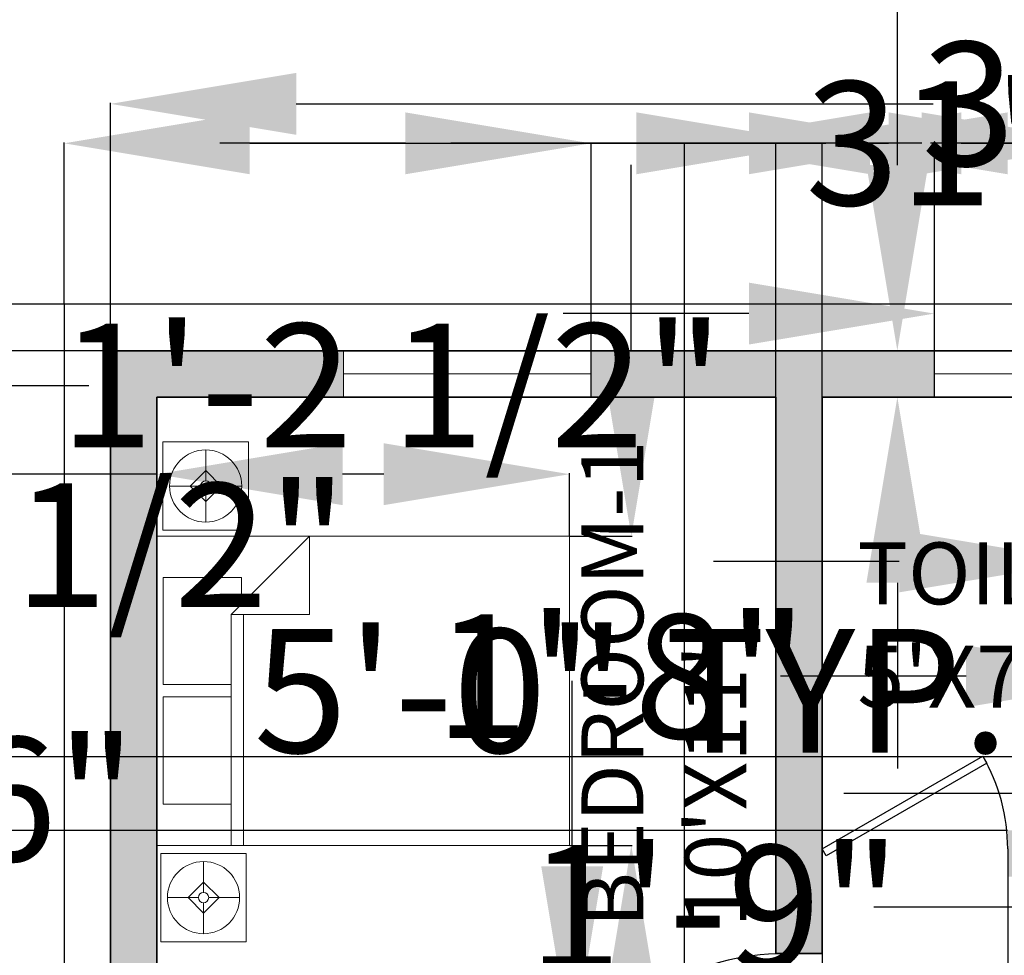
# Model space of a CAD drawing. Units: inches. Extents: x 2838 to 4029, y 1041 to 1915.
# Tile 7 of 16: x 3250 to 3441, y 1554 to 1735. Entities that reach past the tile are written whole.
import ezdxf

# ---------------------------------------------------------------- set-up
doc = ezdxf.new("R2010")
doc.units = ezdxf.units.IN
doc.header["$MEASUREMENT"] = 0
for name, color, linetype, lineweight in [('A-ANNO-DIMS', 2, 'Continuous', 18), ('A-AREA-IDEN', 7, 'Continuous', 18), ('A-DOOR', 3, 'Continuous', 25), ('A-FLOR', 7, 'Continuous', 25), ('A-FURN', 8, 'Continuous', 18), ('A-GLAZ', 4, 'Continuous', 18), ('A-REFR', 8, 'Continuous', 13), ('A-WALL', 7, 'Continuous', 35), ('A-WALL-PATT', 252, 'Continuous', 13)]:
    doc.layers.add(name, color=color, linetype=linetype, lineweight=lineweight)
doc.styles.get("Standard").update_dxf_attribs({"font": 'arial.ttf'})
doc.dimstyles.get("Standard").update_dxf_attribs({"dimtxt": 24, "dimasz": 36, "dimexe": 0.18, "dimexo": 0.0625, "dimgap": 0.09, "dimtad": 0, "dimtih": 1, "dimtoh": 1, "dimdec": 0, "dimzin": 0, "dimdsep": 46, "dimlunit": 3, "dimtxsty": 'Standard', "dimcen": 0.09, "dimadec": 0, "dimazin": 0, "dimtfac": 1, "dimtdec": 0, "dimtofl": 0, "dimtmove": 0, "dimatfit": 3, "dimfxl": 1, "dimtolj": 1, "dimtzin": 0, "dimarcsym": 0})

# ---------------------------------------------------------------- blocks, each defined once
blk = doc.blocks.new('*U2')
for p, q in [((0, 0), (0, -6)), ((40, 0), (40, -6))]:
    blk.add_line(p, q)
blk.add_lwpolyline([(0, 0), (34.64, 20), (35.52, 18.48), (0.87, -1.52)], close=True)
blk.add_arc((0, 0), 40, 0, 30)
blk = doc.blocks.new('*U3')
for p, q in [((-40, 0), (-40, 6)), ((0, 0), (0, 6))]:
    blk.add_line(p, q)
blk.add_lwpolyline([(0, 0), (-20, -34.64), (-21.52, -33.77), (-1.52, 0.88)], close=True)
blk.add_arc((0, 0), 40, 180, 240)
blk = doc.blocks.new('Bed - Queen')
for p, q in [((0, -80.00003), (0, 0)), ((0, 0), (59.99999, 0)), ((59.99999, 0), (59.99999, -80.00003)), ((7.99999, -1.2), (28.79998, -1.2)), ((7.99999, -14.4), (7.99999, -1.2)), ((28.79998, -1.2), (28.79998, -14.4)), ((31.19999, -1.2), (51.99999, -1.2)), ((31.19999, -14.4), (31.19999, -1.2)), ((51.99999, -1.2), (51.99999, -16.4)), ((0, -14.4), (44.8, -14.4)), ((59.99999, -29.6), (44.8, -14.4)), ((44.8, -14.4), (44.8, -29.6)), ((44.8, -16.8), (0, -16.8)), ((51.99999, -16.4), (46.79936, -16.4)), ((44.8, -29.6), (59.99999, -29.6)), ((59.99999, -80.00003), (0, -80.00003))]:
    blk.add_line(p, q)
blk = doc.blocks.new('*D18')
at = {"layer": 'A-ANNO-DIMS', "color": 0, "lineweight": -2, "transparency": 16777216}
for p, q in [((3267.73, 1671.36), (3267.73, 1719.35)), ((3303.73, 1719.17), (3427.28, 1719.17)), ((3591.73, 1719.17), (3468.18, 1719.17)), ((3627.73, 1671.36), (3627.73, 1719.35))]:
    blk.add_line(p, q, dxfattribs=at)
at = {"layer": 'A-ANNO-DIMS', "color": 0, "transparency": 16777216}
for points in [[(3303.73, 1725.17), (3303.73, 1713.17), (3267.73, 1719.17)], [(3591.73, 1725.17), (3591.73, 1713.17), (3627.73, 1719.17)]]:
    blk.add_solid(points, dxfattribs=at)
at = {"layer": 'Defpoints', "color": 0, "transparency": 16777216}
for p in [(3267.73, 1719.17), (3267.73, 1671.3), (3627.73, 1671.3)]:
    blk.add_point(p, dxfattribs=at)
at = {"layer": 'A-ANNO-DIMS', "color": 0, "transparency": 16777216, "insert": (3447.73, 1719.17), "char_height": 24, "attachment_point": 5}
blk.add_mtext("\\A1;30'", dxfattribs=at)
blk = doc.blocks.new('WIN-48')
blk.add_line((4.5, 48), (4.5, 0))
blk.add_lwpolyline([(0, 48), (9, 48), (9, 0), (0, 0)], close=True)
blk = doc.blocks.new('WIN-24-VENT')
for p, q in [((24, 9), (24, 0)), ((24, 4.5), (0, 4.5))]:
    blk.add_line(p, q)
blk.add_lwpolyline([(48, 0), (0, 0), (0, 9), (48, 9)])
blk = doc.blocks.new('Lamp - Table')
for p, q in [((0, 7), (0, 1)), ((0, 3), (-3, 0)), ((3, 0), (0, 3)), ((-1, 0), (-7, 0)), ((-3, 0), (0, -3)), ((0, -3), (3, 0)), ((1, 0), (7, 0)), ((0, -1), (0, -7))]:
    blk.add_line(p, q)
for radius in [7, 1]:
    blk.add_circle((0, 0), radius)
blk = doc.blocks.new('NIGHTSTAND-WITH-LAMP')
blk.add_lwpolyline([(0, 17.15), (16.57, 17.15), (16.57, 0), (0, 0)], close=True)
blk.add_blockref('Lamp - Table', (8.28, 8.57))
blk = doc.blocks.new('*D35')
at = {"layer": 'A-ANNO-DIMS', "color": 0, "lineweight": -2, "transparency": 16777216}
for p, q in [((3480.45, 1632.93), (3480.45, 1668.93)), ((3481.89, 1596.93), (3480.27, 1596.93)), ((3481.89, 1586.93), (3480.27, 1586.93)), ((3480.45, 1550.93), (3480.45, 1514.93)), ((3480.45, 1514.93), (3444.45, 1514.93))]:
    blk.add_line(p, q, dxfattribs=at)
at = {"layer": 'A-ANNO-DIMS', "color": 0, "transparency": 16777216}
for points in [[(3474.45, 1632.93), (3486.45, 1632.93), (3480.45, 1596.93)], [(3474.45, 1550.93), (3486.45, 1550.93), (3480.45, 1586.93)]]:
    blk.add_solid(points, dxfattribs=at)
at = {"layer": 'Defpoints', "color": 0, "transparency": 16777216}
for p in [(3481.95, 1596.93), (3480.45, 1586.93), (3481.95, 1586.93)]:
    blk.add_point(p, dxfattribs=at)
at = {"layer": 'A-ANNO-DIMS', "color": 0, "transparency": 16777216, "insert": (3365.58, 1514.93), "char_height": 24, "attachment_point": 5}
blk.add_mtext('\\A1;TAP 0\'-10"', dxfattribs=at)
blk = doc.blocks.new('*D36')
at = {"layer": 'A-ANNO-DIMS', "color": 0, "lineweight": -2, "transparency": 16777216}
for p, q in [((3481.95, 1586.87), (3481.95, 1585.25)), ((3488.45, 1586.87), (3488.45, 1585.25)), ((3445.95, 1585.43), (3409.95, 1585.43)), ((3524.45, 1585.43), (3560.45, 1585.43))]:
    blk.add_line(p, q, dxfattribs=at)
at = {"layer": 'A-ANNO-DIMS', "color": 0, "transparency": 16777216}
for points in [[(3445.95, 1591.43), (3445.95, 1579.43), (3481.95, 1585.43)], [(3524.45, 1591.43), (3524.45, 1579.43), (3488.45, 1585.43)]]:
    blk.add_solid(points, dxfattribs=at)
at = {"layer": 'Defpoints', "color": 0, "transparency": 16777216}
for p in [(3481.95, 1586.93), (3488.45, 1586.93), (3488.45, 1585.43)]:
    blk.add_point(p, dxfattribs=at)
at = {"layer": 'A-ANNO-DIMS', "color": 0, "transparency": 16777216, "insert": (3620.4, 1585.43), "char_height": 24, "attachment_point": 5}
blk.add_mtext('\\A1;0\'-6 1/2"', dxfattribs=at)
blk = doc.blocks.new('*D37')
at = {"layer": 'A-ANNO-DIMS', "color": 0, "lineweight": -2, "transparency": 16777216}
for p, q in [((3276.73, 1647.36), (3240.73, 1647.36)), ((3276.73, 1635.42), (3276.73, 1647.54)), ((3320.73, 1647.36), (3312.73, 1647.36)), ((3356.73, 1635.42), (3356.73, 1647.54))]:
    blk.add_line(p, q, dxfattribs=at)
at = {"layer": 'A-ANNO-DIMS', "color": 0, "transparency": 16777216}
for points in [[(3312.73, 1653.36), (3312.73, 1641.36), (3276.73, 1647.36)], [(3320.73, 1653.36), (3320.73, 1641.36), (3356.73, 1647.36)]]:
    blk.add_solid(points, dxfattribs=at)
at = {"layer": 'Defpoints', "color": 0, "transparency": 16777216}
for p in [(3276.73, 1647.36), (3276.73, 1635.36), (3356.73, 1635.36)]:
    blk.add_point(p, dxfattribs=at)
at = {"layer": 'A-ANNO-DIMS', "color": 0, "transparency": 16777216, "insert": (3064.12, 1647.36), "char_height": 24, "attachment_point": 5}
blk.add_mtext('\\A1;QUEEN BED 6\'-8" TYP.', dxfattribs=at)
blk = doc.blocks.new('*D38')
at = {"layer": 'A-ANNO-DIMS', "color": 0, "lineweight": -2, "transparency": 16777216}
for p, q in [((3368.73, 1671.36), (3368.73, 1707.36)), ((3356.79, 1635.36), (3368.91, 1635.36)), ((3356.79, 1575.36), (3368.91, 1575.36)), ((3368.73, 1539.36), (3368.73, 1503.36))]:
    blk.add_line(p, q, dxfattribs=at)
at = {"layer": 'A-ANNO-DIMS', "color": 0, "transparency": 16777216}
for points in [[(3362.73, 1671.36), (3374.73, 1671.36), (3368.73, 1635.36)], [(3362.73, 1539.36), (3374.73, 1539.36), (3368.73, 1575.36)]]:
    blk.add_solid(points, dxfattribs=at)
at = {"layer": 'Defpoints', "color": 0, "transparency": 16777216}
for p in [(3356.73, 1635.36), (3368.73, 1635.36), (3356.73, 1575.36)]:
    blk.add_point(p, dxfattribs=at)
at = {"layer": 'A-ANNO-DIMS', "color": 0, "transparency": 16777216, "insert": (3368.73, 1605.36), "char_height": 24, "attachment_point": 5}
blk.add_mtext('\\A1;5\'-0" TYP.', dxfattribs=at)
blk = doc.blocks.new('*D39')
at = {"layer": 'A-ANNO-DIMS', "color": 0, "lineweight": -2, "transparency": 16777216}
for p, q in [((3427.52, 1671.36), (3427.52, 1678.68)), ((3475.52, 1671.36), (3475.52, 1678.68)), ((3391.52, 1678.5), (3355.52, 1678.5)), ((3511.52, 1678.5), (3547.52, 1678.5))]:
    blk.add_line(p, q, dxfattribs=at)
at = {"layer": 'A-ANNO-DIMS', "color": 0, "transparency": 16777216}
for points in [[(3391.52, 1684.5), (3391.52, 1672.5), (3427.52, 1678.5)], [(3511.52, 1684.5), (3511.52, 1672.5), (3475.52, 1678.5)]]:
    blk.add_solid(points, dxfattribs=at)
at = {"layer": 'Defpoints', "color": 0, "transparency": 16777216}
for p in [(3475.52, 1678.5), (3427.52, 1671.3), (3475.52, 1671.3)]:
    blk.add_point(p, dxfattribs=at)
at = {"layer": 'A-ANNO-DIMS', "color": 0, "transparency": 16777216, "insert": (3732.24, 1678.5), "char_height": 24, "attachment_point": 5}
blk.add_mtext('\\A1;VENT BLOCK 4\'-0" TYP.', dxfattribs=at)
blk = doc.blocks.new('*D40')
at = {"layer": 'A-ANNO-DIMS', "color": 0, "lineweight": -2, "transparency": 16777216}
for p, q in [((3420.32, 1707.3), (3420.32, 1743.3)), ((3420.32, 1743.3), (3456.32, 1743.3)), ((3427.46, 1671.3), (3420.14, 1671.3)), ((3427.46, 1662.3), (3420.14, 1662.3)), ((3420.32, 1626.3), (3420.32, 1590.3))]:
    blk.add_line(p, q, dxfattribs=at)
at = {"layer": 'A-ANNO-DIMS', "color": 0, "transparency": 16777216}
for points in [[(3414.32, 1707.3), (3426.32, 1707.3), (3420.32, 1671.3)], [(3414.32, 1626.3), (3426.32, 1626.3), (3420.32, 1662.3)]]:
    blk.add_solid(points, dxfattribs=at)
at = {"layer": 'Defpoints', "color": 0, "transparency": 16777216}
for p in [(3420.32, 1671.3), (3427.52, 1671.3), (3427.52, 1662.3)]:
    blk.add_point(p, dxfattribs=at)
at = {"layer": 'A-ANNO-DIMS', "color": 0, "transparency": 16777216, "insert": (3529.56, 1743.3), "char_height": 24, "attachment_point": 5}
blk.add_mtext('\\A1;0\'-9" TYP.', dxfattribs=at)
blk = doc.blocks.new('*D41')
at = {"layer": 'A-ANNO-DIMS', "color": 0, "lineweight": -2, "transparency": 16777216}
for p, q in [((3284.24, 1506.2), (3284.24, 1496.56)), ((3347.73, 1506.2), (3347.73, 1496.56)), ((3248.24, 1496.74), (3212.24, 1496.74)), ((3383.73, 1496.74), (3419.73, 1496.74))]:
    blk.add_line(p, q, dxfattribs=at)
at = {"layer": 'A-ANNO-DIMS', "color": 0, "transparency": 16777216}
for points in [[(3248.24, 1502.74), (3248.24, 1490.74), (3284.24, 1496.74)], [(3383.73, 1502.74), (3383.73, 1490.74), (3347.73, 1496.74)]]:
    blk.add_solid(points, dxfattribs=at)
at = {"layer": 'Defpoints', "color": 0, "transparency": 16777216}
for p in [(3284.24, 1506.26), (3347.73, 1506.26), (3347.73, 1496.74)]:
    blk.add_point(p, dxfattribs=at)
at = {"layer": 'A-ANNO-DIMS', "color": 0, "transparency": 16777216, "insert": (3624.81, 1496.74), "char_height": 24, "attachment_point": 5}
blk.add_mtext('\\A1;WARDROBE 5\'-3 1/2" TYP.', dxfattribs=at)
blk = doc.blocks.new('*D42')
at = {"layer": 'A-ANNO-DIMS', "color": 0, "lineweight": -2, "transparency": 16777216}
for p, q in [((3357.26, 1571.32), (3357.26, 1607.32)), ((3347.8, 1535.32), (3357.44, 1535.32)), ((3347.8, 1506.26), (3357.44, 1506.26)), ((3357.26, 1470.26), (3357.26, 1434.26))]:
    blk.add_line(p, q, dxfattribs=at)
at = {"layer": 'A-ANNO-DIMS', "color": 0, "transparency": 16777216}
for points in [[(3351.26, 1571.32), (3363.26, 1571.32), (3357.26, 1535.32)], [(3351.26, 1470.26), (3363.26, 1470.26), (3357.26, 1506.26)]]:
    blk.add_solid(points, dxfattribs=at)
at = {"layer": 'Defpoints', "color": 0, "transparency": 16777216}
for p in [(3347.73, 1535.32), (3357.26, 1535.32), (3347.73, 1506.26)]:
    blk.add_point(p, dxfattribs=at)
at = {"layer": 'A-ANNO-DIMS', "color": 0, "transparency": 16777216, "insert": (3357.26, 1520.79), "char_height": 24, "attachment_point": 5}
blk.add_mtext('\\A1;2\'-5" TYP.', dxfattribs=at)
blk = doc.blocks.new('*D45')
at = {"layer": 'A-ANNO-DIMS', "color": 0, "lineweight": -2, "transparency": 16777216}
for p, q in [((3456.69, 1635.35), (3456.69, 1630.27)), ((3489.73, 1635.35), (3489.73, 1630.27)), ((3420.69, 1630.45), (3384.69, 1630.45)), ((3525.73, 1630.45), (3561.73, 1630.45))]:
    blk.add_line(p, q, dxfattribs=at)
at = {"layer": 'A-ANNO-DIMS', "color": 0, "transparency": 16777216}
for points in [[(3420.69, 1636.45), (3420.69, 1624.45), (3456.69, 1630.45)], [(3525.73, 1636.45), (3525.73, 1624.45), (3489.73, 1630.45)]]:
    blk.add_solid(points, dxfattribs=at)
at = {"layer": 'Defpoints', "color": 0, "transparency": 16777216}
for p in [(3456.69, 1635.41), (3489.73, 1635.41), (3489.73, 1630.45)]:
    blk.add_point(p, dxfattribs=at)
at = {"layer": 'A-ANNO-DIMS', "color": 0, "transparency": 16777216, "insert": (3626.8, 1630.45), "char_height": 24, "attachment_point": 5}
blk.add_mtext('\\A1;WC 2\'-9"', dxfattribs=at)
blk = doc.blocks.new('*D46')
at = {"layer": 'A-ANNO-DIMS', "color": 0, "lineweight": -2, "transparency": 16777216}
for p, q in [((3451.73, 1692.41), (3451.73, 1728.41)), ((3456.62, 1656.41), (3451.55, 1656.41)), ((3456.62, 1635.41), (3451.55, 1635.41)), ((3451.73, 1599.41), (3451.73, 1563.41)), ((3451.73, 1563.41), (3415.73, 1563.41))]:
    blk.add_line(p, q, dxfattribs=at)
at = {"layer": 'A-ANNO-DIMS', "color": 0, "transparency": 16777216}
for points in [[(3445.73, 1692.41), (3457.73, 1692.41), (3451.73, 1656.41)], [(3445.73, 1599.41), (3457.73, 1599.41), (3451.73, 1635.41)]]:
    blk.add_solid(points, dxfattribs=at)
at = {"layer": 'Defpoints', "color": 0, "transparency": 16777216}
for p in [(3456.69, 1656.41), (3451.73, 1635.41), (3456.69, 1635.41)]:
    blk.add_point(p, dxfattribs=at)
at = {"layer": 'A-ANNO-DIMS', "color": 0, "transparency": 16777216, "insert": (3384.87, 1563.41), "char_height": 24, "attachment_point": 5}
blk.add_mtext('\\A1;1\'-9"', dxfattribs=at)
blk = doc.blocks.new('*D48')
at = {"layer": 'A-ANNO-DIMS', "color": 0, "lineweight": -2, "transparency": 16777216}
for p, q in [((3433.65, 1608.18), (3397.65, 1608.18)), ((3469.65, 1604.56), (3469.65, 1608.36)), ((3489.78, 1604.56), (3489.78, 1608.36)), ((3525.78, 1608.18), (3561.78, 1608.18))]:
    blk.add_line(p, q, dxfattribs=at)
at = {"layer": 'A-ANNO-DIMS', "color": 0, "transparency": 16777216}
for points in [[(3433.65, 1614.18), (3433.65, 1602.18), (3469.65, 1608.18)], [(3525.78, 1614.18), (3525.78, 1602.18), (3489.78, 1608.18)]]:
    blk.add_solid(points, dxfattribs=at)
at = {"layer": 'Defpoints', "color": 0, "transparency": 16777216}
for p in [(3469.65, 1608.18), (3469.65, 1604.5), (3489.78, 1604.5)]:
    blk.add_point(p, dxfattribs=at)
at = {"layer": 'A-ANNO-DIMS', "color": 0, "transparency": 16777216, "insert": (3366.79, 1608.18), "char_height": 24, "attachment_point": 5}
blk.add_mtext('\\A1;1\'-8"', dxfattribs=at)
blk = doc.blocks.new('*D55')
at = {"layer": 'A-ANNO-DIMS', "color": 0, "lineweight": -2, "transparency": 16777216}
for p, q in [((3491.76, 1499.78), (3455.76, 1499.78)), ((3527.76, 1494.67), (3527.76, 1499.96)), ((3562.26, 1494.67), (3562.26, 1499.96)), ((3598.26, 1499.78), (3634.26, 1499.78))]:
    blk.add_line(p, q, dxfattribs=at)
at = {"layer": 'A-ANNO-DIMS', "color": 0, "transparency": 16777216}
for points in [[(3491.76, 1505.78), (3491.76, 1493.78), (3527.76, 1499.78)], [(3598.26, 1505.78), (3598.26, 1493.78), (3562.26, 1499.78)]]:
    blk.add_solid(points, dxfattribs=at)
at = {"layer": 'Defpoints', "color": 0, "transparency": 16777216}
for p in [(3527.76, 1499.78), (3527.76, 1494.6), (3562.26, 1494.6)]:
    blk.add_point(p, dxfattribs=at)
at = {"layer": 'A-ANNO-DIMS', "color": 0, "transparency": 16777216, "insert": (3260.33, 1499.78), "char_height": 24, "attachment_point": 5}
blk.add_mtext('\\A1;BASE CABINET 2\'-10 1/2"', dxfattribs=at)
blk = doc.blocks.new('*D64')
at = {"layer": 'A-ANNO-DIMS', "color": 0, "lineweight": -2, "transparency": 16777216}
for p, q in [((3076.99, 1633.6), (3040.99, 1633.6)), ((3112.99, 1623.27), (3112.99, 1633.78)), ((3117.35, 1626.21), (3117.35, 1633.78)), ((3153.35, 1633.6), (3189.35, 1633.6))]:
    blk.add_line(p, q, dxfattribs=at)
at = {"layer": 'A-ANNO-DIMS', "color": 0, "transparency": 16777216}
for points in [[(3076.99, 1639.6), (3076.99, 1627.6), (3112.99, 1633.6)], [(3153.35, 1639.6), (3153.35, 1627.6), (3117.35, 1633.6)]]:
    blk.add_solid(points, dxfattribs=at)
at = {"layer": 'Defpoints', "color": 0, "transparency": 16777216}
for p in [(3117.35, 1633.6), (3117.35, 1626.15), (3112.99, 1623.2)]:
    blk.add_point(p, dxfattribs=at)
at = {"layer": 'A-ANNO-DIMS', "color": 0, "transparency": 16777216, "insert": (3249.3, 1633.6), "char_height": 24, "attachment_point": 5}
blk.add_mtext('\\A1;0\'-4 1/2"', dxfattribs=at)
blk = doc.blocks.new('*D67')
at = {"layer": 'A-ANNO-DIMS', "color": 0, "lineweight": -2, "transparency": 16777216}
for p, q in [((3258.67, 1680.3), (3227.33, 1680.3)), ((3227.51, 1644.3), (3227.51, 1409.15)), ((3227.51, 1149.3), (3227.51, 1384.45)), ((3329.6, 1113.3), (3227.33, 1113.3))]:
    blk.add_line(p, q, dxfattribs=at)
at = {"layer": 'A-ANNO-DIMS', "color": 0, "transparency": 16777216}
for points in [[(3221.51, 1644.3), (3233.51, 1644.3), (3227.51, 1680.3)], [(3221.51, 1149.3), (3233.51, 1149.3), (3227.51, 1113.3)]]:
    blk.add_solid(points, dxfattribs=at)
at = {"layer": 'Defpoints', "color": 0, "transparency": 16777216}
for p in [(3227.51, 1680.3), (3258.73, 1680.3), (3329.66, 1113.3)]:
    blk.add_point(p, dxfattribs=at)
at = {"layer": 'A-ANNO-DIMS', "color": 0, "transparency": 16777216, "insert": (3227.51, 1396.8), "char_height": 24, "attachment_point": 5}
blk.add_mtext('\\A1;47\'-3"', dxfattribs=at)
blk = doc.blocks.new('*D68')
at = {"layer": 'A-ANNO-DIMS', "color": 0, "lineweight": -2, "transparency": 16777216}
for p, q in [((3258.73, 1680.36), (3258.73, 1711.7)), ((3294.73, 1711.52), (3406.43, 1711.52)), ((3600.73, 1711.52), (3489.04, 1711.52)), ((3636.73, 1680.36), (3636.73, 1711.7))]:
    blk.add_line(p, q, dxfattribs=at)
at = {"layer": 'A-ANNO-DIMS', "color": 0, "transparency": 16777216}
for points in [[(3294.73, 1717.52), (3294.73, 1705.52), (3258.73, 1711.52)], [(3600.73, 1717.52), (3600.73, 1705.52), (3636.73, 1711.52)]]:
    blk.add_solid(points, dxfattribs=at)
at = {"layer": 'Defpoints', "color": 0, "transparency": 16777216}
for p in [(3636.73, 1711.52), (3258.73, 1680.3), (3636.73, 1680.3)]:
    blk.add_point(p, dxfattribs=at)
at = {"layer": 'A-ANNO-DIMS', "color": 0, "transparency": 16777216, "insert": (3447.73, 1711.52), "char_height": 24, "attachment_point": 5}
blk.add_mtext('\\A1;31\'-6"', dxfattribs=at)
blk = doc.blocks.new('*D73')
at = {"layer": 'A-ANNO-DIMS', "color": 0, "lineweight": -2, "transparency": 16777216}
for p, q in [((3425.038746, 1711.522346), (3389.038746, 1711.522346)), ((3461.038746, 1200.359846), (3461.038746, 1711.702346)), ((3618.731626, 1200.359846), (3618.731626, 1711.702346)), ((3654.731626, 1711.522346), (3690.731626, 1711.522346))]:
    blk.add_line(p, q, dxfattribs=at)
at = {"layer": 'A-ANNO-DIMS', "color": 0, "transparency": 16777216}
for points in [[(3425.038746, 1717.522346), (3425.038746, 1705.522346), (3461.038746, 1711.522346)], [(3654.731626, 1717.522346), (3654.731626, 1705.522346), (3618.731626, 1711.522346)]]:
    blk.add_solid(points, dxfattribs=at)
at = {"layer": 'Defpoints', "color": 0, "transparency": 16777216}
for p in [(3618.731626, 1711.522346), (3461.038746, 1200.297346), (3618.731626, 1200.297346)]:
    blk.add_point(p, dxfattribs=at)
at = {"layer": 'A-ANNO-DIMS', "color": 0, "transparency": 16777216, "insert": (3539.885186, 1711.522346), "char_height": 24, "attachment_point": 5}
blk.add_mtext('\\A1;13\'-1 1/2"', dxfattribs=at)
blk = doc.blocks.new('*D77')
at = {"layer": 'A-ANNO-DIMS', "color": 0, "lineweight": -2, "transparency": 16777216}
for p, q in [((3267.67, 1671.3), (3227.33, 1671.3)), ((3227.51, 1635.3), (3227.51, 1596.69)), ((3227.51, 1533.39), (3227.51, 1572)), ((3276.67, 1497.39), (3227.33, 1497.39))]:
    blk.add_line(p, q, dxfattribs=at)
at = {"layer": 'A-ANNO-DIMS', "color": 0, "transparency": 16777216}
for points in [[(3221.51, 1635.3), (3233.51, 1635.3), (3227.51, 1671.3)], [(3221.51, 1533.39), (3233.51, 1533.39), (3227.51, 1497.39)]]:
    blk.add_solid(points, dxfattribs=at)
at = {"layer": 'Defpoints', "color": 0, "transparency": 16777216}
for p in [(3227.51, 1671.3), (3267.73, 1671.3), (3276.73, 1497.39)]:
    blk.add_point(p, dxfattribs=at)
at = {"layer": 'A-ANNO-DIMS', "color": 0, "transparency": 16777216, "insert": (3227.51, 1584.35), "char_height": 24, "attachment_point": 5}
blk.add_mtext('\\A1;14\'-6"', dxfattribs=at)
blk = doc.blocks.new('*D79')
at = {"layer": 'A-ANNO-DIMS', "color": 0, "lineweight": -2, "transparency": 16777216}
for p, q in [((3379.05, 1400.64), (3379.05, 1711.7)), ((3415.05, 1711.52), (3418.63, 1711.52)), ((3454.63, 1398.31), (3454.63, 1711.7)), ((3454.63, 1711.52), (3490.63, 1711.52))]:
    blk.add_line(p, q, dxfattribs=at)
at = {"layer": 'A-ANNO-DIMS', "color": 0, "transparency": 16777216}
for points in [[(3415.05, 1717.52), (3415.05, 1705.52), (3379.05, 1711.52)], [(3418.63, 1717.52), (3418.63, 1705.52), (3454.63, 1711.52)]]:
    blk.add_solid(points, dxfattribs=at)
at = {"layer": 'Defpoints', "color": 0, "transparency": 16777216}
for p in [(3454.63, 1711.52), (3379.05, 1400.57), (3454.63, 1398.25)]:
    blk.add_point(p, dxfattribs=at)
at = {"layer": 'A-ANNO-DIMS', "color": 0, "transparency": 16777216, "insert": (3550.65, 1711.52), "char_height": 24, "attachment_point": 5}
blk.add_mtext('\\A1;6\'-3 1/2"', dxfattribs=at)
blk = doc.blocks.new('*D80')
at = {"layer": 'A-ANNO-DIMS', "color": 0, "lineweight": -2, "transparency": 16777216}
for p, q in [((3324.91, 1711.52), (3288.91, 1711.52)), ((3360.91, 1662.36), (3360.91, 1711.7)), ((3396.73, 1662.36), (3396.73, 1711.7)), ((3432.73, 1711.52), (3468.73, 1711.52))]:
    blk.add_line(p, q, dxfattribs=at)
at = {"layer": 'A-ANNO-DIMS', "color": 0, "transparency": 16777216}
for points in [[(3324.91, 1717.52), (3324.91, 1705.52), (3360.91, 1711.52)], [(3432.73, 1717.52), (3432.73, 1705.52), (3396.73, 1711.52)]]:
    blk.add_solid(points, dxfattribs=at)
at = {"layer": 'Defpoints', "color": 0, "transparency": 16777216}
for p in [(3396.73, 1711.52), (3360.91, 1662.3), (3396.73, 1662.3)]:
    blk.add_point(p, dxfattribs=at)
at = {"layer": 'A-ANNO-DIMS', "color": 0, "transparency": 16777216, "insert": (3500.71, 1711.52), "char_height": 24, "attachment_point": 5}
blk.add_mtext('\\A1;3\'-0"', dxfattribs=at)
blk = doc.blocks.new('*D82')
at = {"layer": 'A-ANNO-DIMS', "color": 0, "lineweight": -2, "transparency": 16777216}
for p, q in [((3405.73, 1573.06), (3405.73, 1081.89)), ((3441.73, 1569.23), (3441.73, 1081.89)), ((3369.73, 1082.07), (3333.73, 1082.07)), ((3477.73, 1082.07), (3513.73, 1082.07))]:
    blk.add_line(p, q, dxfattribs=at)
at = {"layer": 'A-ANNO-DIMS', "color": 0, "transparency": 16777216}
for points in [[(3369.73, 1088.07), (3369.73, 1076.07), (3405.73, 1082.07)], [(3477.73, 1088.07), (3477.73, 1076.07), (3441.73, 1082.07)]]:
    blk.add_solid(points, dxfattribs=at)
at = {"layer": 'Defpoints', "color": 0, "transparency": 16777216}
for p in [(3405.73, 1573.12), (3441.73, 1569.3), (3441.73, 1082.07)]:
    blk.add_point(p, dxfattribs=at)
at = {"layer": 'A-ANNO-DIMS', "color": 0, "transparency": 16777216, "insert": (3545.71, 1082.07), "char_height": 24, "attachment_point": 5}
blk.add_mtext('\\A1;3\'-0"', dxfattribs=at)
blk = doc.blocks.new('*D83')
at = {"layer": 'A-ANNO-DIMS', "color": 0, "lineweight": -2, "transparency": 16777216}
for p, q in [((3405.73, 1662.36), (3405.73, 1711.7)), ((3441.73, 1711.52), (3453.73, 1711.52)), ((3489.73, 1662.36), (3489.73, 1711.7)), ((3489.73, 1711.52), (3525.73, 1711.52))]:
    blk.add_line(p, q, dxfattribs=at)
at = {"layer": 'A-ANNO-DIMS', "color": 0, "transparency": 16777216}
for points in [[(3441.73, 1717.52), (3441.73, 1705.52), (3405.73, 1711.52)], [(3453.73, 1717.52), (3453.73, 1705.52), (3489.73, 1711.52)]]:
    blk.add_solid(points, dxfattribs=at)
at = {"layer": 'Defpoints', "color": 0, "transparency": 16777216}
for p in [(3489.73, 1711.52), (3405.73, 1662.3), (3489.73, 1662.3)]:
    blk.add_point(p, dxfattribs=at)
at = {"layer": 'A-ANNO-DIMS', "color": 0, "transparency": 16777216, "insert": (3557.62, 1711.52), "char_height": 24, "attachment_point": 5}
blk.add_mtext('\\A1;7\'-0"', dxfattribs=at)
blk = doc.blocks.new('*D85')
at = {"layer": 'A-ANNO-DIMS', "color": 0, "lineweight": -2, "transparency": 16777216}
for p, q in [((3369.73, 1711.52), (3333.73, 1711.52)), ((3405.73, 1662.36), (3405.73, 1711.7)), ((3427.52, 1662.36), (3427.52, 1711.7)), ((3463.52, 1711.52), (3499.52, 1711.52))]:
    blk.add_line(p, q, dxfattribs=at)
at = {"layer": 'A-ANNO-DIMS', "color": 0, "transparency": 16777216}
for points in [[(3369.73, 1717.52), (3369.73, 1705.52), (3405.73, 1711.52)], [(3463.52, 1717.52), (3463.52, 1705.52), (3427.52, 1711.52)]]:
    blk.add_solid(points, dxfattribs=at)
at = {"layer": 'Defpoints', "color": 0, "transparency": 16777216}
for p in [(3427.52, 1711.52), (3405.73, 1662.3), (3427.52, 1662.3)]:
    blk.add_point(p, dxfattribs=at)
at = {"layer": 'A-ANNO-DIMS', "color": 0, "transparency": 16777216, "insert": (3539.7, 1711.52), "char_height": 24, "attachment_point": 5}
blk.add_mtext('\\A1;1\'-10"', dxfattribs=at)
blk = doc.blocks.new('*D86')
at = {"layer": 'A-ANNO-DIMS', "color": 0, "lineweight": -2, "transparency": 16777216}
for p, q in [((3391.52, 1711.52), (3355.52, 1711.52)), ((3427.52, 1671.36), (3427.52, 1711.7)), ((3451.52, 1671.36), (3451.52, 1711.7)), ((3487.52, 1711.52), (3523.52, 1711.52))]:
    blk.add_line(p, q, dxfattribs=at)
at = {"layer": 'A-ANNO-DIMS', "color": 0, "transparency": 16777216}
for points in [[(3391.52, 1717.52), (3391.52, 1705.52), (3427.52, 1711.52)], [(3487.52, 1717.52), (3487.52, 1705.52), (3451.52, 1711.52)]]:
    blk.add_solid(points, dxfattribs=at)
at = {"layer": 'Defpoints', "color": 0, "transparency": 16777216}
for p in [(3451.52, 1711.52), (3427.52, 1671.3), (3451.52, 1671.3)]:
    blk.add_point(p, dxfattribs=at)
at = {"layer": 'A-ANNO-DIMS', "color": 0, "transparency": 16777216, "insert": (3555.72, 1711.52), "char_height": 24, "attachment_point": 5}
blk.add_mtext('\\A1;2\'-0"', dxfattribs=at)
blk = doc.blocks.new('*D91')
at = {"layer": 'A-ANNO-DIMS', "color": 0, "lineweight": -2, "transparency": 16777216}
for p, q in [((3227.506626, 1533.394218), (3227.506626, 1569.394218)), ((3522.669126, 1497.394218), (3227.326626, 1497.394218)), ((3522.669126, 1461.394218), (3227.326626, 1461.394218)), ((3227.506626, 1425.394218), (3227.506626, 1389.394218))]:
    blk.add_line(p, q, dxfattribs=at)
at = {"layer": 'A-ANNO-DIMS', "color": 0, "transparency": 16777216}
for points in [[(3221.506626, 1533.394218), (3233.506626, 1533.394218), (3227.506626, 1497.394218)], [(3221.506626, 1425.394218), (3233.506626, 1425.394218), (3227.506626, 1461.394218)]]:
    blk.add_solid(points, dxfattribs=at)
at = {"layer": 'Defpoints', "color": 0, "transparency": 16777216}
for p in [(3522.731626, 1497.394218), (3227.506626, 1461.394218), (3522.731626, 1461.394218)]:
    blk.add_point(p, dxfattribs=at)
at = {"layer": 'A-ANNO-DIMS', "color": 0, "transparency": 16777216, "insert": (3227.506626, 1479.394218), "char_height": 24, "attachment_point": 5}
blk.add_mtext('\\A1;3\'-0"', dxfattribs=at)
blk = doc.blocks.new('*D96')
at = {"layer": 'A-ANNO-DIMS', "color": 0, "lineweight": -2, "transparency": 16777216}
for p, q in [((3462.73, 1711.52), (3426.73, 1711.52)), ((3498.73, 1662.36), (3498.73, 1711.7)), ((3546.42, 1662.36), (3546.42, 1711.7)), ((3582.42, 1711.52), (3618.42, 1711.52))]:
    blk.add_line(p, q, dxfattribs=at)
at = {"layer": 'A-ANNO-DIMS', "color": 0, "transparency": 16777216}
for points in [[(3462.73, 1717.52), (3462.73, 1705.52), (3498.73, 1711.52)], [(3582.42, 1717.52), (3582.42, 1705.52), (3546.42, 1711.52)]]:
    blk.add_solid(points, dxfattribs=at)
at = {"layer": 'Defpoints', "color": 0, "transparency": 16777216}
for p in [(3546.42, 1711.52), (3498.73, 1662.3), (3546.42, 1662.3)]:
    blk.add_point(p, dxfattribs=at)
at = {"layer": 'A-ANNO-DIMS', "color": 0, "transparency": 16777216, "insert": (3687.68, 1711.52), "char_height": 24, "attachment_point": 5}
blk.add_mtext('\\A1;3\'-11 1/2"', dxfattribs=at)
blk = doc.blocks.new('*D101')
at = {"layer": 'A-ANNO-DIMS', "color": 0, "lineweight": -2, "transparency": 16777216}
for p, q in [((3425.04, 1711.52), (3389.04, 1711.52)), ((3461.04, 1200.36), (3461.04, 1711.7)), ((3486.18, 1200.36), (3486.18, 1711.7)), ((3522.18, 1711.52), (3558.18, 1711.52))]:
    blk.add_line(p, q, dxfattribs=at)
at = {"layer": 'A-ANNO-DIMS', "color": 0, "transparency": 16777216}
for points in [[(3425.04, 1717.52), (3425.04, 1705.52), (3461.04, 1711.52)], [(3522.18, 1717.52), (3522.18, 1705.52), (3486.18, 1711.52)]]:
    blk.add_solid(points, dxfattribs=at)
at = {"layer": 'Defpoints', "color": 0, "transparency": 16777216}
for p in [(3486.18, 1711.52), (3461.04, 1200.3), (3486.18, 1200.3)]:
    blk.add_point(p, dxfattribs=at)
at = {"layer": 'A-ANNO-DIMS', "color": 0, "transparency": 16777216, "insert": (3590.37, 1711.52), "char_height": 24, "attachment_point": 5}
blk.add_mtext('\\A1;2\'-1"', dxfattribs=at)
blk = doc.blocks.new('*D103')
at = {"layer": 'A-ANNO-DIMS', "color": 0, "lineweight": -2, "transparency": 16777216}
for p, q in [((3227.51, 1628.55), (3227.51, 1664.55)), ((3227.51, 1664.55), (3263.51, 1664.55)), ((3469.64, 1592.55), (3227.33, 1592.55)), ((3441.67, 1578.3), (3227.33, 1578.3)), ((3227.51, 1542.3), (3227.51, 1506.3))]:
    blk.add_line(p, q, dxfattribs=at)
at = {"layer": 'A-ANNO-DIMS', "color": 0, "transparency": 16777216}
for points in [[(3221.51, 1628.55), (3233.51, 1628.55), (3227.51, 1592.55)], [(3221.51, 1542.3), (3233.51, 1542.3), (3227.51, 1578.3)]]:
    blk.add_solid(points, dxfattribs=at)
at = {"layer": 'Defpoints', "color": 0, "transparency": 16777216}
for p in [(3227.51, 1592.55), (3469.7, 1592.55), (3441.73, 1578.3)]:
    blk.add_point(p, dxfattribs=at)
at = {"layer": 'A-ANNO-DIMS', "color": 0, "transparency": 16777216, "insert": (3322.33, 1664.55), "char_height": 24, "attachment_point": 5}
blk.add_mtext('\\A1;1\'-2 1/2"', dxfattribs=at)

msp = doc.modelspace()

# ---------------------------------------------------------------- hatches: boundary and pattern name
at = {"layer": 'A-WALL-PATT'}
h = msp.add_hatch(color=256, dxfattribs=at)
h.dxf.hatch_style = 1
h.paths.add_polyline_path([(3405.73, 1506.39), (3297.05, 1506.39), (3297.01, 1506.26), (3297.01, 1506.39), (3286.16, 1506.39), (3286.11, 1506.26), (3286.11, 1506.39), (3276.73, 1506.39), (3276.73, 1535.45), (3276.73, 1662.3), (3312.91, 1662.3), (3312.91, 1671.3), (3267.73, 1671.3), (3267.73, 1480.17), (3276.73, 1480.17), (3276.73, 1497.39), (3405.73, 1497.39)])
h = msp.add_hatch(color=256, dxfattribs=at)
h.dxf.hatch_style = 1
h.paths.add_polyline_path([(3427.52, 1671.3), (3360.91, 1671.3), (3360.91, 1662.3), (3396.73, 1662.3), (3396.73, 1554.39), (3397.12, 1554.39, -0.007312), (3398.53, 1554.41), (3405.73, 1554.41), (3405.73, 1662.3), (3427.52, 1662.3)])
h.paths.add_polyline_path([(3546.42, 1671.3), (3451.52, 1671.3), (3451.52, 1662.3), (3489.73, 1662.3), (3489.73, 1592.86, -0.016107), (3489.73, 1591.9), (3489.73, 1578.3), (3441.73, 1578.3), (3441.73, 1569.3), (3489.73, 1569.3), (3489.73, 1554.41), (3498.73, 1554.41), (3498.73, 1662.3), (3546.42, 1662.3)])
h.paths.add_polyline_path([(3627.73, 1671.3), (3594.42, 1671.3), (3594.42, 1662.3), (3618.73, 1662.3), (3618.73, 1634.03), (3627.73, 1634.03)])
h.paths.add_polyline_path([(3627.73, 1586.03), (3618.73, 1586.03), (3618.73, 1506.39), (3545.12, 1506.39), (3489.73, 1506.39), (3489.73, 1497.39), (3513.73, 1497.39), (3618.73, 1497.39), (3618.73, 1469.85), (3627.73, 1469.85)])
h.paths.add_polyline_path([(3627.73, 1421.85), (3618.73, 1421.85), (3618.73, 1378.73), (3522.73, 1378.73), (3513.73, 1378.73), (3461.04, 1378.73), (3461.04, 1369.73), (3513.73, 1369.73), (3618.73, 1369.73), (3618.73, 1320.94), (3627.73, 1320.94)])
h.paths.add_polyline_path([(3627.73, 1272.94), (3618.73, 1272.94), (3618.73, 1200.3), (3599.07, 1200.3), (3599.07, 1191.3), (3627.73, 1191.3)])
h.paths.add_polyline_path([(3551.07, 1200.3), (3510.18, 1200.3), (3510.18, 1191.3), (3551.07, 1191.3)])
h.paths.add_polyline_path([(3486.18, 1200.3), (3461.04, 1200.3), (3461.04, 1398.25), (3454.63, 1398.25), (3454.63, 1200.3), (3432.45, 1200.3), (3432.45, 1191.3), (3486.18, 1191.3)])
h.paths.add_polyline_path([(3300.73, 1200.3), (3276.73, 1200.3), (3276.73, 1391.57), (3331.05, 1391.57), (3331.05, 1400.57), (3276.73, 1400.57), (3276.73, 1432.17), (3267.73, 1432.17), (3267.73, 1191.3), (3300.73, 1191.3)])

# ---------------------------------------------------------------- linework, layer by layer
at = {"layer": 'A-FLOR'}
msp.add_lwpolyline([(3527.95, 1182.3), (3636.73, 1182.3), (3636.73, 1680.3), (3258.73, 1680.3), (3258.73, 1182.3), (3267.73, 1182.3)], dxfattribs=at)
at = {"layer": 'A-REFR'}
msp.add_point((3258.73, 1671.3), dxfattribs=at)
at = {"layer": 'A-WALL'}
for p, q in [((3627.73, 1671.3), (3267.73, 1671.3)), ((3267.73, 1671.3), (3267.73, 1191.3)), ((3276.73, 1662.3), (3276.73, 1506.39)), ((3396.73, 1662.3), (3276.73, 1662.3)), ((3276.73, 1506.39), (3276.73, 1662.3)), ((3276.73, 1662.3), (3312.91, 1662.3)), ((3312.91, 1662.3), (3360.91, 1662.3)), ((3360.91, 1662.3), (3396.73, 1662.3)), ((3396.73, 1662.3), (3396.73, 1554.39)), ((3396.73, 1662.3), (3396.73, 1554.39)), ((3405.73, 1662.3), (3405.73, 1554.39)), ((3489.73, 1662.3), (3405.73, 1662.3)), ((3405.73, 1554.39), (3405.73, 1662.3)), ((3405.73, 1662.3), (3489.73, 1662.3)), ((3405.73, 1554.39), (3396.73, 1554.39)), ((3396.73, 1554.39), (3405.73, 1554.39))]:
    msp.add_line(p, q, dxfattribs=at)
msp.add_lwpolyline([(3372.73, 1191.3), (3627.73, 1191.3), (3627.73, 1671.3), (3267.73, 1671.3), (3267.73, 1191.3), (3300.73, 1191.3)], dxfattribs=at)

# ---------------------------------------------------------------- block references
at = {"layer": 'A-DOOR', "xscale": 0.899795500672641, "yscale": 0.899795500672641, "zscale": 0.899795500672641}
msp.add_blockref('*U2', (3405.73, 1574.7), dxfattribs=at)
at = {"layer": 'A-DOOR', "xscale": 1.200513446172712, "yscale": 1.200513446172712, "zscale": 1.200513446172712, "rotation": 270}
msp.add_blockref('*U3', (3398.53, 1506.39), dxfattribs=at)
at = {"layer": 'A-FURN'}
for p in [(3277.9, 1636.5), (3277.49, 1556.69)]:
    msp.add_blockref('NIGHTSTAND-WITH-LAMP', p, dxfattribs=at)
at = {"layer": 'A-FURN', "rotation": 90}
msp.add_blockref('Bed - Queen', (3276.73, 1575.36), dxfattribs=at)
at = {"layer": 'A-GLAZ', "rotation": 269.9999999999973}
msp.add_blockref('WIN-48', (3312.91, 1671.3), dxfattribs=at)
at = {"layer": 'A-GLAZ'}
msp.add_blockref('WIN-24-VENT', (3427.52, 1662.3), dxfattribs=at)

# ---------------------------------------------------------------- texts
at = {"layer": 'A-AREA-IDEN', "insert": (3391.06, 1559.47), "char_height": 12, "attachment_point": 7, "rotation": 90}
msp.add_mtext_dynamic_manual_height_columns("BEDROOM-1\\P10'X11'", width=64.6015, gutter_width=1, heights=[0], dxfattribs=at)
at = {"layer": 'A-AREA-IDEN', "insert": (3412.59, 1634.12), "char_height": 12, "attachment_point": 1}
msp.add_mtext_dynamic_manual_height_columns("TOILET\\P5'X7'", width=64.6015, gutter_width=1, heights=[0], dxfattribs=at)

# ---------------------------------------------------------------- dimensions: what is measured, and where the dimension line sits
at = {"layer": 'A-ANNO-DIMS'}
for base, p1, p2, angle, text, picture, middle in [((3420.32, 1671.3), (3427.52, 1662.3), (3427.52, 1671.3), 90, '<> TYP.', '*D40', (3529.56, 1743.3)), ((3276.73, 1647.36), (3356.73, 1635.36), (3276.73, 1635.36), 180, 'QUEEN BED <> TYP.', '*D37', (3064.12, 1647.36)), ((3368.73, 1635.36), (3356.73, 1575.36), (3356.73, 1635.36), 90, '<> TYP.', '*D38', (3368.73, 1605.36)), ((3480.45, 1586.93), (3481.95, 1596.93), (3481.95, 1586.93), 270, 'TAP <>', '*D35', (3365.58, 1514.93)), ((3357.26, 1535.32), (3347.73, 1506.26), (3347.73, 1535.32), 90, '<> TYP.', '*D42', (3357.26, 1520.79)), ((3527.76, 1499.78), (3562.26, 1494.6), (3527.76, 1494.6), 180, 'BASE CABINET <>', '*D55', (3260.33, 1499.78))]:
    dim = msp.add_linear_dim(base=base, p1=p1, p2=p2, angle=angle, text=text, dimstyle='Standard', override={"dimdec": 1, "dimlfac": 1, "dimrnd": 0, "dimzin": 1, "dimdsep": 46, "dimlunit": 4, "dimfrac": 2}, dxfattribs=at)
    dim.commit()
    dim.dimension.update_dxf_attribs({"geometry": picture, "text_midpoint": middle})
for base, p1, p2, text, picture, middle in [((3475.52, 1678.5), (3427.52, 1671.3), (3475.52, 1671.3), 'VENT BLOCK <> TYP.', '*D39', (3732.24, 1678.5)), ((3489.73, 1630.45), (3456.69, 1635.41), (3489.73, 1635.41), 'WC <>', '*D45', (3626.8, 1630.45)), ((3347.73, 1496.74), (3284.24, 1506.26), (3347.73, 1506.26), 'WARDROBE <> TYP.', '*D41', (3624.81, 1496.74))]:
    dim = msp.add_linear_dim(base=base, p1=p1, p2=p2, text=text, dimstyle='Standard', override={"dimdec": 1, "dimlfac": 1, "dimrnd": 0, "dimzin": 1, "dimdsep": 46, "dimlunit": 4, "dimfrac": 2}, dxfattribs=at)
    dim.commit()
    dim.dimension.update_dxf_attribs({"geometry": picture, "text_midpoint": middle})
for base, p1, p2, override, picture, middle in [((3454.63, 1711.52), (3379.05, 1400.57), (3454.63, 1398.25), {"dimdec": 1, "dimlfac": 1, "dimrnd": 0, "dimzin": 1, "dimdsep": 46, "dimlunit": 4, "dimfrac": 2}, '*D79', (3550.65, 1711.52)), ((3618.73, 1711.52), (3461.04, 1200.3), (3618.73, 1200.3), {"dimdec": 1, "dimlfac": 1, "dimrnd": 0, "dimzin": 1, "dimdsep": 46, "dimlunit": 4, "dimfrac": 2}, '*D73', (3539.89, 1711.52)), ((3546.42, 1711.52), (3498.73, 1662.3), (3546.42, 1662.3), {"dimdec": 1, "dimlfac": 1, "dimrnd": 0, "dimzin": 1, "dimdsep": 46, "dimlunit": 4, "dimfrac": 2}, '*D96', (3687.68, 1711.52)), ((3267.73, 1719.17), (3627.73, 1671.3), (3267.73, 1671.3), {"dimclrd": 0, "dimclre": 0, "dimclrt": 0}, '*D18', (3447.73, 1719.17)), ((3636.73, 1711.52), (3258.73, 1680.3), (3636.73, 1680.3), {"dimdec": 1, "dimlfac": 1, "dimrnd": 0, "dimzin": 1, "dimdsep": 46, "dimlunit": 4, "dimfrac": 2}, '*D68', (3447.73, 1711.52)), ((3396.73, 1711.52), (3360.91, 1662.3), (3396.73, 1662.3), {"dimdec": 1, "dimlfac": 1, "dimrnd": 0, "dimzin": 1, "dimdsep": 46, "dimlunit": 4, "dimfrac": 2}, '*D80', (3500.71, 1711.52)), ((3427.52, 1711.52), (3405.73, 1662.3), (3427.52, 1662.3), {"dimdec": 1, "dimlfac": 1, "dimrnd": 0, "dimzin": 1, "dimdsep": 46, "dimlunit": 4, "dimfrac": 2}, '*D85', (3539.7, 1711.52)), ((3451.52, 1711.52), (3427.52, 1671.3), (3451.52, 1671.3), {"dimdec": 1, "dimlfac": 1, "dimrnd": 0, "dimzin": 1, "dimdsep": 46, "dimlunit": 4, "dimfrac": 2}, '*D86', (3555.72, 1711.52)), ((3486.18, 1711.52), (3461.04, 1200.3), (3486.18, 1200.3), {"dimdec": 1, "dimlfac": 1, "dimrnd": 0, "dimzin": 1, "dimdsep": 46, "dimlunit": 4, "dimfrac": 2}, '*D101', (3590.37, 1711.52)), ((3489.73, 1711.52), (3405.73, 1662.3), (3489.73, 1662.3), {"dimdec": 1, "dimlfac": 1, "dimrnd": 0, "dimzin": 1, "dimdsep": 46, "dimlunit": 4, "dimfrac": 2}, '*D83', (3557.62, 1711.52)), ((3117.35, 1633.6), (3112.99, 1623.2), (3117.35, 1626.15), {"dimdec": 1, "dimlfac": 1, "dimrnd": 0, "dimzin": 1, "dimdsep": 46, "dimlunit": 4, "dimfrac": 2}, '*D64', (3249.3, 1633.6)), ((3488.45, 1585.43), (3481.95, 1586.93), (3488.45, 1586.93), {"dimdec": 1, "dimlfac": 1, "dimrnd": 0, "dimzin": 1, "dimdsep": 46, "dimlunit": 4, "dimfrac": 2}, '*D36', (3620.4, 1585.43)), ((3441.73, 1082.07), (3405.73, 1573.12), (3441.73, 1569.3), {"dimdec": 1, "dimlfac": 1, "dimrnd": 0, "dimzin": 1, "dimdsep": 46, "dimlunit": 4, "dimfrac": 2}, '*D82', (3545.71, 1082.07))]:
    dim = msp.add_linear_dim(base=base, p1=p1, p2=p2, dimstyle='Standard', override=override, dxfattribs=at)
    dim.commit()
    dim.dimension.update_dxf_attribs({"geometry": picture, "text_midpoint": middle})
for base, p1, p2, angle, picture, middle in [((3451.73, 1635.41), (3456.69, 1656.41), (3456.69, 1635.41), 270, '*D46', (3384.87, 1563.41)), ((3227.5066, 1592.5486), (3441.7316, 1578.2973), (3469.6999, 1592.5486), 90, '*D103', (3322.3279, 1664.5486)), ((3227.51, 1680.3), (3329.66, 1113.3), (3258.73, 1680.3), 90, '*D67', (3227.51, 1396.8)), ((3227.51, 1671.3), (3276.73, 1497.39), (3267.73, 1671.3), 90, '*D77', (3227.51, 1584.35)), ((3469.65, 1608.18), (3489.78, 1604.5), (3469.65, 1604.5), 180, '*D48', (3366.79, 1608.18)), ((3227.51, 1461.39), (3522.73, 1497.39), (3522.73, 1461.39), 90, '*D91', (3227.51, 1479.39))]:
    dim = msp.add_linear_dim(base=base, p1=p1, p2=p2, angle=angle, dimstyle='Standard', override={"dimdec": 1, "dimlfac": 1, "dimrnd": 0, "dimzin": 1, "dimdsep": 46, "dimlunit": 4, "dimfrac": 2}, dxfattribs=at)
    dim.commit()
    dim.dimension.update_dxf_attribs({"geometry": picture, "text_midpoint": middle})

doc.saveas('drawing.dxf')
